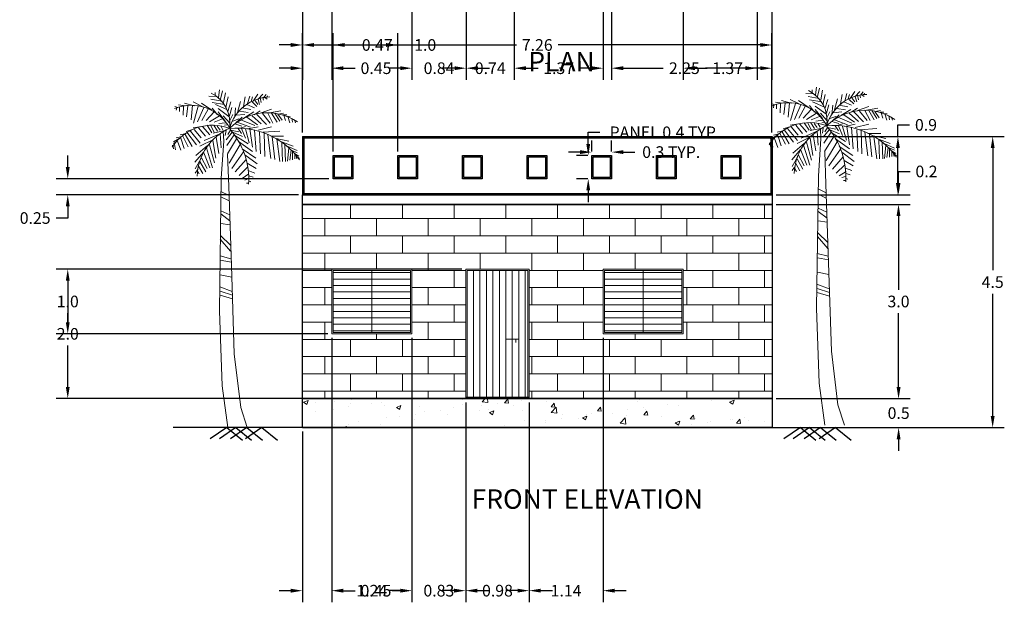
# Model space of a CAD drawing. Units: metres. Extents: x 40.9 to 56.1, y -1.4 to 24.2.
# Tile 1 of 7: x 40.9 to 56.1, y -1.4 to 7.6. Entities that reach past the tile are written whole.
import ezdxf

# ---------------------------------------------------------------- set-up
doc = ezdxf.new("R2010")
doc.units = ezdxf.units.M
doc.header["$MEASUREMENT"] = 0
for name, color, linetype, lineweight in [('A-ANNO-DIMS', 2, 'Continuous', 18), ('A-ANNO-TITL', 7, 'Continuous', 25), ('A-ELEV', 7, 'Continuous', 30), ('A-ELEV-DOOR', 3, 'Continuous', 18), ('A-ELEV-GLAZ', 4, 'Continuous', 18), ('A-ELEV-GRND', 7, 'Continuous', 25), ('A-ELEV-PATT', 252, 'Continuous', 13), ('L-PLNT', 94, 'Continuous', 13)]:
    doc.layers.add(name, color=color, linetype=linetype, lineweight=lineweight)
doc.styles.get("Standard").update_dxf_attribs({"font": 'arial.ttf'})
doc.dimstyles.get("Standard").update_dxf_attribs({"dimtxt": 0.18, "dimasz": 0.18, "dimexe": 0.18, "dimexo": 0.0625, "dimgap": 0.09, "dimtad": 0, "dimtih": 1, "dimtoh": 1, "dimdec": 1, "dimzin": 0, "dimdsep": 46, "dimtxsty": 'Standard', "dimcen": 0.09, "dimadec": 0, "dimazin": 0, "dimtfac": 1, "dimtdec": 1, "dimtofl": 0, "dimtmove": 0, "dimatfit": 3, "dimfxl": 1, "dimtolj": 1, "dimtzin": 0, "dimarcsym": 0})

# ---------------------------------------------------------------- blocks, each defined once
blk = doc.blocks.new('*U47')
for p, q in [((-190.5, 5071.872), (-190.5, 5027.8284)), ((-141.4018, 4996.3578), (-126.6698, 5109.6418)), ((-111.9378, 4971.1864), (-82.4738, 5097.0688)), ((-386.8928, 4857.877), (-524.3576, 4927.1174)), ((-170.8658, 5008.9308), (-288.6964, 5015.23)), ((-87.4014, 4939.7158), (-254.3302, 4971.1864)), ((-48.1076, 4889.3476), (-234.696, 4920.8182)), ((-62.8396, 4920.8182), (-33.401, 5065.5982)), ((-28.4734, 4845.2786), (5.8928, 5002.657)), ((0.9652, 4782.3374), (45.1612, 4927.1174)), ((148.2598, 4769.7644), (192.4558, 4933.4166)), ((236.6518, 4857.877), (261.1882, 5002.657)), ((300.4566, 4901.946), (334.8228, 5015.23)), ((354.4824, 4933.4166), (374.1166, 5002.657)), ((369.2144, 4927.1174), (437.9468, 4857.877)), ((383.9464, 4939.7158), (452.6788, 5046.7006)), ((408.4828, 4952.2888), (452.6788, 4889.3476)), ((457.581, 4971.1864), (531.2156, 5046.7006)), ((457.581, 4964.8872), (482.1174, 4889.3476)), ((491.9472, 4990.0586), (506.6792, 4920.8182)), ((531.2156, 4990.0586), (541.0454, 4952.2888)), ((541.0454, 4990.0586), (580.3138, 5040.4014)), ((560.6796, 4996.3578), (595.0458, 4971.1864)), ((590.1436, 4996.3578), (599.948, 5021.5292)), ((-755.1166, 4845.2786), (-799.3126, 4857.877)), ((-769.8486, 4839.0048), (-779.653, 4801.235)), ((-642.1882, 4870.4754), (-745.2868, 4883.0484)), ((-730.5802, 4845.2786), (-730.5802, 4782.3374)), ((-671.6522, 4864.1762), (-676.5544, 4725.6954)), ((-509.6256, 4870.4754), (-656.9202, 4908.2452)), ((-602.9198, 4870.4754), (-622.554, 4700.524)), ((-534.1874, 4876.7492), (-553.8216, 4656.455)), ((-445.7954, 4864.1762), (-519.4554, 4606.1122)), ((-362.331, 4845.2786), (-460.5274, 4624.9844)), ((-239.5982, 4801.235), (-396.6972, 4908.2452)), ((-298.5262, 4820.1072), (-391.795, 4643.882)), ((-205.232, 4776.0636), (-327.9648, 4643.882)), ((-156.1338, 4731.9946), (-234.696, 4832.7056)), ((-13.7414, 4813.808), (-185.5978, 4889.3476)), ((-146.304, 4826.4064), (15.6972, 4706.8232)), ((-146.304, 4776.0636), (-38.3032, 4637.5828)), ((25.527, 4719.3962), (59.8932, 4845.2786)), ((104.0892, 4700.524), (118.8212, 4839.0048)), ((177.7238, 4788.6366), (310.2864, 4769.7644)), ((217.0176, 4839.0048), (349.5802, 4813.808)), ((241.554, 4681.6518), (393.7508, 4776.0636)), ((285.75, 4889.3476), (403.5806, 4839.0048)), ((398.653, 4731.9946), (491.9472, 4794.9358)), ((491.9472, 4757.166), (663.7782, 4820.1072)), ((629.412, 4763.4652), (801.2684, 4794.9358)), ((-126.6698, 4719.3962), (-278.8666, 4624.9844)), ((-82.4738, 4669.0534), (-205.232, 4618.6852)), ((-67.7672, 4719.3962), (30.4292, 4606.1122)), ((25.527, 4637.5828), (74.6252, 4738.2938)), ((74.6252, 4637.5828), (167.894, 4669.0534)), ((123.7234, 4725.6954), (256.286, 4738.2938)), ((123.7234, 4612.4114), (217.0176, 4694.2248)), ((143.3576, 4618.6852), (344.6526, 4543.171)), ((197.358, 4656.455), (408.4828, 4568.3424)), ((285.75, 4694.2248), (447.7512, 4580.9408)), ((369.2144, 4719.3962), (506.6792, 4593.5138)), ((437.9468, 4738.2938), (585.2414, 4587.2146)), ((526.3134, 4750.8668), (639.2418, 4606.1122)), ((604.8756, 4757.166), (683.4378, 4606.1122)), ((663.7782, 4757.166), (747.2426, 4618.6852)), ((712.8764, 4757.166), (786.5364, 4637.5828)), ((757.0724, 4744.593), (820.9026, 4650.1812)), ((761.9746, 4744.593), (840.5368, 4757.166)), ((825.8048, 4731.9946), (894.5372, 4731.9946)), ((850.3666, 4725.6954), (874.903, 4643.882)), ((904.367, 4713.1224), (943.6354, 4706.8232)), ((909.2692, 4706.8232), (938.7332, 4612.4114)), ((968.1972, 4681.6518), (978.0016, 4618.6852)), ((1012.3678, 4643.882), (1022.1976, 4612.4114)), ((-534.1874, 4511.7004), (-632.3838, 4480.2298)), ((-563.6514, 4486.529), (-416.3314, 4303.9792)), ((-396.6972, 4555.744), (-524.3576, 4536.8718)), ((-509.6256, 4511.7004), (-401.6248, 4385.818)), ((-440.8932, 4536.8718), (-337.7946, 4410.9894)), ((-381.9652, 4555.744), (-273.9644, 4429.8616)), ((-313.2328, 4574.6416), (-239.5982, 4461.3322)), ((-259.2324, 4574.6416), (-205.232, 4467.6314)), ((-43.2054, 4492.8028), (-219.964, 4455.0584)), ((-210.1342, 4574.6416), (-156.1338, 4486.529)), ((-161.036, 4562.0432), (-116.84, 4499.102)), ((-33.401, 4612.4114), (-136.4996, 4599.813)), ((-102.1334, 4555.744), (-72.6694, 4505.4012)), ((-67.7672, 4480.2298), (-60.3504, 4333.0876)), ((-8.8392, 4580.9408), (-48.1076, 4574.6416)), ((-23.5712, 4492.8028), (-38.3032, 4417.2886)), ((40.259, 4499.102), (0.9652, 4436.1608)), ((40.259, 4499.102), (167.894, 4473.9306)), ((104.0892, 4593.5138), (212.09, 4562.0432)), ((158.0896, 4524.2734), (207.1878, 4448.7592)), ((187.5536, 4530.5726), (266.0904, 4555.744)), ((207.1878, 4524.2734), (266.0904, 4379.5188)), ((266.0904, 4517.9996), (325.0184, 4310.2784)), ((300.4566, 4517.9996), (457.581, 4549.4702)), ((334.8228, 4517.9996), (374.1166, 4241.038)), ((403.5806, 4499.102), (428.117, 4178.0968)), ((457.581, 4499.102), (663.7782, 4549.4702)), ((531.2156, 4467.6314), (786.5364, 4486.529)), ((-735.4824, 4373.2196), (-823.849, 4322.8768)), ((-696.1886, 4404.6902), (-779.653, 4385.818)), ((-760.0188, 4335.4498), (-710.9206, 4196.969)), ((-637.286, 4448.7592), (-720.7504, 4429.8616)), ((-710.9206, 4379.5188), (-661.8224, 4222.1658)), ((-681.4566, 4410.9894), (-598.0176, 4247.3372)), ((-647.0904, 4436.1608), (-539.0896, 4253.6364)), ((-617.6518, 4467.6314), (-475.2594, 4278.8078)), ((-215.0364, 4360.6212), (-421.259, 4259.9102)), ((-107.0356, 4448.7592), (-357.4288, 4341.749)), ((-224.8662, 4341.749), (-180.6702, 4077.3858)), ((-175.768, 4392.0918), (-136.4996, 4146.6262)), ((-116.84, 4442.46), (-102.1334, 4234.7388)), ((64.7954, 4467.6314), (-23.5712, 4354.3474)), ((94.2594, 4429.8616), (-13.7414, 4266.2094)), ((133.5278, 4366.9204), (-3.937, 4140.327)), ((74.6252, 4467.6314), (221.9198, 4404.6902)), ((108.9914, 4417.2886), (310.2864, 4291.4062)), ((162.9918, 4329.1506), (374.1166, 4178.0968)), ((482.1174, 4467.6314), (496.8494, 4140.327)), ((550.8752, 4455.0584), (560.6796, 4102.5572)), ((604.8756, 4429.8616), (649.0716, 4071.0866)), ((649.0716, 4410.9894), (845.439, 4410.9894)), ((673.608, 4398.391), (712.8764, 4058.5136)), ((732.5106, 4373.2196), (924.0012, 4335.4498)), ((742.3404, 4366.9204), (786.5364, 4027.043)), ((786.5364, 4335.4498), (987.8314, 4259.9102)), ((-828.7512, 4266.2094), (-843.4832, 4266.2094)), ((-828.7512, 4259.9102), (-823.849, 4215.8666)), ((-789.4828, 4316.5776), (-823.849, 4297.68)), ((-804.2148, 4285.107), (-789.4828, 4203.2682)), ((-362.331, 4171.7976), (-499.8212, 4014.4446)), ((-308.3306, 4266.2094), (-485.0892, 4115.1556)), ((-323.0626, 4234.7388), (-229.7684, 3932.6312)), ((-278.8666, 4278.8078), (-200.3298, 4008.1454)), ((187.5536, 4285.107), (20.6248, 4001.8462)), ((236.6518, 4171.7976), (59.8932, 3920.0328)), ((217.0176, 4215.8666), (423.2148, 4077.3858)), ((816.0004, 4310.2784), (825.8048, 4027.043)), ((865.0732, 4285.107), (874.903, 4027.043)), ((899.4648, 4259.9102), (1051.6616, 4190.6952)), ((924.0012, 4228.4396), (904.367, 4033.3168)), ((958.3674, 4196.969), (938.7332, 4045.9152)), ((963.2696, 4196.969), (1051.6616, 4159.2246)), ((978.0016, 4178.0968), (978.0016, 4052.2144)), ((-406.527, 4064.7874), (-494.8936, 3913.7336)), ((-421.259, 4027.043), (-332.8924, 3869.69)), ((-396.6972, 4083.685), (-313.2328, 3920.0328)), ((-362.331, 4159.2246), (-273.9644, 3932.6312)), ((275.9202, 4058.5136), (113.8936, 3869.69)), ((256.286, 4127.754), (442.849, 3989.2732)), ((1007.4656, 4146.6262), (1076.198, 4108.8564)), ((1012.3678, 4134.0278), (1012.3678, 4064.7874)), ((1036.9296, 4108.8564), (1046.734, 4064.7874)), ((1046.734, 4102.5572), (1086.0278, 4071.0866)), ((-460.5274, 3901.1606), (-494.8936, 3850.7924)), ((-455.6252, 3875.9638), (-431.0888, 3838.2194)), ((-440.8932, 3957.8026), (-377.063, 3844.4932)), ((300.4566, 3938.905), (172.8216, 3813.0226)), ((290.6522, 4001.8462), (428.117, 3920.0328)), ((310.2864, 3888.5622), (408.4828, 3850.7924)), ((320.1162, 3838.2194), (217.0176, 3768.979)), ((310.2864, 3762.6798), (256.286, 3743.7822)), ((315.1886, 3731.2092), (349.5802, 3718.6108)), ((320.1162, 3806.7488), (383.9464, 3787.8512)), ((315.1886, 3699.7386), (280.8224, 3699.7386)), ((-103.6574, 3572.383), (19.1262, 3511.8294)), ((-103.6574, 3493.6938), (19.1262, 3433.1402)), ((-103.6574, 3281.807), (28.5496, 3221.2534)), ((-103.6574, 3233.3692), (33.274, 3130.4484)), ((-103.6574, 3088.0812), (33.274, 3069.9202)), ((-113.1062, 2851.9882), (42.7228, 2670.3782)), ((-108.3818, 2906.4712), (42.7228, 2761.1832)), ((-117.8306, 2597.7342), (47.4472, 2555.3416)), ((-113.1062, 2531.1354), (56.896, 2500.8586)), ((-113.1062, 2313.2034), (61.6204, 2276.8814)), ((-122.555, 2131.5934), (66.3448, 2058.9494)), ((-117.8306, 2064.9946), (71.0438, 2004.4664)), ((-117.8306, 2004.4664), (71.0438, 1949.9834))]:
    blk.add_line(p, q)
for points in [[(-60.0202, 4332.0462), (-98.552, 3772.027), (-126.6952, 1768.7036), (-84.455, 631.6726), (0, 0)], [(-2.9464, 4136.3392), (14.0716, 3645.7128), (56.3118, 2454.529), (98.552, 1118.9716), (197.104, 306.8066), (295.656, 0)]]:
    blk.add_lwpolyline(points)
for centre, radius, start, end in [((-468.0458, 4608.7792), 500.7615, 350.285, 64.11229), ((650.113, 4357.8018), 645.0437, 91.40319, 163.882), ((-552.1452, 4218.7876), 657.8234, 27.67115, 112.5305), ((601.6498, 3945.6614), 817.5767, 56.19272, 134.3213), ((-235.1786, 3853.9928), 721.0064, 68.38311, 147.5322), ((365.6076, 3769.1822), 831.8901, 113.7592, 177.4133), ((148.0312, 3371.0372), 1159.2273, 35.98777, 95.82273), ((-833.12, 3757.2442), 1150.8562, 356.1943, 41.37848)]:
    blk.add_arc(centre, radius, start, end)
blk = doc.blocks.new('*D48')
at = {"layer": 'A-ANNO-DIMS', "color": 0, "lineweight": -2, "transparency": 16777216}
for p, q in [((54.473, 1.933), (54.473, 2.113)), ((52.578, 1.753), (54.653, 1.753)), ((52.578, 1.303), (54.653, 1.303)), ((54.473, 1.123), (54.473, 0.943))]:
    blk.add_line(p, q, dxfattribs=at)
at = {"layer": 'A-ANNO-DIMS', "color": 0, "transparency": 16777216}
for points in [[(54.443, 1.933), (54.503, 1.933), (54.473, 1.753)], [(54.443, 1.123), (54.503, 1.123), (54.473, 1.303)]]:
    blk.add_solid(points, dxfattribs=at)
at = {"layer": 'Defpoints', "color": 0, "transparency": 16777216}
for p in [(52.515, 1.753), (52.515, 1.303), (54.473, 1.303)]:
    blk.add_point(p, dxfattribs=at)
at = {"layer": 'A-ANNO-DIMS', "color": 0, "transparency": 16777216, "insert": (54.473, 1.528), "char_height": 0.18, "attachment_point": 5}
blk.add_mtext('\\A1;0.5', dxfattribs=at)
blk = doc.blocks.new('*D49')
at = {"layer": 'A-ANNO-DIMS', "color": 0, "lineweight": -2, "transparency": 16777216}
for p, q in [((52.578, 4.753), (54.651, 4.753)), ((54.471, 4.573), (54.471, 3.435)), ((54.471, 1.933), (54.471, 3.071)), ((52.578, 1.753), (54.651, 1.753))]:
    blk.add_line(p, q, dxfattribs=at)
at = {"layer": 'A-ANNO-DIMS', "color": 0, "transparency": 16777216}
for points in [[(54.441, 4.573), (54.501, 4.573), (54.471, 4.753)], [(54.441, 1.933), (54.501, 1.933), (54.471, 1.753)]]:
    blk.add_solid(points, dxfattribs=at)
at = {"layer": 'Defpoints', "color": 0, "transparency": 16777216}
for p in [(52.515, 4.753), (54.471, 4.753), (52.515, 1.753)]:
    blk.add_point(p, dxfattribs=at)
at = {"layer": 'A-ANNO-DIMS', "color": 0, "transparency": 16777216, "insert": (54.471, 3.253), "char_height": 0.18, "attachment_point": 5}
blk.add_mtext('\\A1;3.0', dxfattribs=at)
blk = doc.blocks.new('*D50')
at = {"layer": 'A-ANNO-DIMS', "color": 0, "lineweight": -2, "transparency": 16777216}
for p, q in [((54.471, 5.083), (54.471, 5.263)), ((54.471, 5.263), (54.651, 5.263)), ((52.578, 4.903), (54.651, 4.903)), ((52.578, 4.753), (54.651, 4.753)), ((54.471, 4.573), (54.471, 4.393))]:
    blk.add_line(p, q, dxfattribs=at)
at = {"layer": 'A-ANNO-DIMS', "color": 0, "transparency": 16777216}
for points in [[(54.441, 5.083), (54.501, 5.083), (54.471, 4.903)], [(54.441, 4.573), (54.501, 4.573), (54.471, 4.753)]]:
    blk.add_solid(points, dxfattribs=at)
at = {"layer": 'Defpoints', "color": 0, "transparency": 16777216}
for p in [(52.515, 4.903), (54.471, 4.903), (52.515, 4.753)]:
    blk.add_point(p, dxfattribs=at)
at = {"layer": 'A-ANNO-DIMS', "color": 0, "transparency": 16777216, "insert": (54.904, 5.263), "char_height": 0.18, "attachment_point": 5}
blk.add_mtext('\\A1;0.2', dxfattribs=at)
blk = doc.blocks.new('*D51')
at = {"layer": 'A-ANNO-DIMS', "color": 0, "lineweight": -2, "transparency": 16777216}
for p, q in [((54.462, 5.803), (54.462, 5.983)), ((54.462, 5.983), (54.642, 5.983)), ((52.578, 5.803), (54.642, 5.803)), ((54.462, 5.083), (54.462, 5.623)), ((52.578, 4.903), (54.642, 4.903))]:
    blk.add_line(p, q, dxfattribs=at)
at = {"layer": 'A-ANNO-DIMS', "color": 0, "transparency": 16777216}
for points in [[(54.432, 5.623), (54.492, 5.623), (54.462, 5.803)], [(54.432, 5.083), (54.492, 5.083), (54.462, 4.903)]]:
    blk.add_solid(points, dxfattribs=at)
at = {"layer": 'Defpoints', "color": 0, "transparency": 16777216}
for p in [(52.515, 5.803), (54.462, 5.803), (52.515, 4.903)]:
    blk.add_point(p, dxfattribs=at)
at = {"layer": 'A-ANNO-DIMS', "color": 0, "transparency": 16777216, "insert": (54.896, 5.983), "char_height": 0.18, "attachment_point": 5}
blk.add_mtext('\\A1;0.9', dxfattribs=at)
blk = doc.blocks.new('PARAPET-FRAMED-PANEL')
for points in [[(0, 0.358), (0.306, 0.358), (0.306, 0), (0, 0)], [(0.02, 0.338), (0.286, 0.338), (0.286, 0.02), (0.02, 0.02)]]:
    blk.add_lwpolyline(points, close=True)
blk = doc.blocks.new('GRADE-MARK-ELEV')
for p, q in [((0.255, 0.195), (0, 0.02)), ((0.396, 0.195), (0.141, 0.02)), ((0.255, 0.195), (0.496, 0)), ((0.566, 0.195), (0.311, 0.02)), ((0.396, 0.195), (0.637, 0)), ((0.799, 0.195), (0.544, 0.02)), ((0.566, 0.195), (0.807, 0)), ((0.799, 0.195), (1.04, 0))]:
    blk.add_line(p, q)
blk = doc.blocks.new('*D77')
at = {"layer": 'A-ANNO-DIMS', "color": 0, "lineweight": -2, "transparency": 16777216}
for p, q in [((49.674, 5.688), (49.674, 5.868)), ((49.674, 5.868), (49.854, 5.868)), ((49.665, 5.508), (49.494, 5.508)), ((49.665, 5.15), (49.494, 5.15)), ((49.674, 4.97), (49.674, 4.79))]:
    blk.add_line(p, q, dxfattribs=at)
at = {"layer": 'A-ANNO-DIMS', "color": 0, "transparency": 16777216}
for points in [[(49.644, 5.688), (49.704, 5.688), (49.674, 5.508)], [(49.644, 4.97), (49.704, 4.97), (49.674, 5.15)]]:
    blk.add_solid(points, dxfattribs=at)
at = {"layer": 'Defpoints', "color": 0, "transparency": 16777216}
for p in [(49.674, 5.508), (49.728, 5.508), (49.728, 5.15)]:
    blk.add_point(p, dxfattribs=at)
at = {"layer": 'A-ANNO-DIMS', "color": 0, "transparency": 16777216, "insert": (50.86, 5.868), "char_height": 0.18, "attachment_point": 5}
blk.add_mtext('\\A1;PANEL 0.4 TYP.', dxfattribs=at)
blk = doc.blocks.new('*D78')
at = {"layer": 'A-ANNO-DIMS', "color": 0, "lineweight": -2, "transparency": 16777216}
for p, q in [((49.728, 5.57), (49.728, 5.742)), ((50.034, 5.57), (50.034, 5.742)), ((49.548, 5.562), (49.368, 5.562)), ((50.214, 5.562), (50.394, 5.562))]:
    blk.add_line(p, q, dxfattribs=at)
at = {"layer": 'A-ANNO-DIMS', "color": 0, "transparency": 16777216}
for points in [[(49.548, 5.592), (49.548, 5.532), (49.728, 5.562)], [(50.214, 5.592), (50.214, 5.532), (50.034, 5.562)]]:
    blk.add_solid(points, dxfattribs=at)
at = {"layer": 'Defpoints', "color": 0, "transparency": 16777216}
for p in [(49.728, 5.508), (50.034, 5.562), (50.034, 5.508)]:
    blk.add_point(p, dxfattribs=at)
at = {"layer": 'A-ANNO-DIMS', "color": 0, "transparency": 16777216, "insert": (50.957, 5.562), "char_height": 0.18, "attachment_point": 5}
blk.add_mtext('\\A1;0.3 TYP.', dxfattribs=at)
blk = doc.blocks.new('*D117')
at = {"layer": 'A-ANNO-DIMS', "color": 0, "lineweight": -2, "transparency": 16777216}
for p, q in [((45.255, 5.866), (45.255, 7.398)), ((52.515, 5.866), (52.515, 7.398)), ((45.435, 7.218), (48.562, 7.218)), ((52.335, 7.218), (49.208, 7.218))]:
    blk.add_line(p, q, dxfattribs=at)
at = {"layer": 'A-ANNO-DIMS', "color": 0, "transparency": 16777216}
for points in [[(45.435, 7.248), (45.435, 7.188), (45.255, 7.218)], [(52.335, 7.248), (52.335, 7.188), (52.515, 7.218)]]:
    blk.add_solid(points, dxfattribs=at)
at = {"layer": 'Defpoints', "color": 0, "transparency": 16777216}
for p in [(52.515, 7.218), (45.255, 5.803), (52.515, 5.803)]:
    blk.add_point(p, dxfattribs=at)
at = {"layer": 'A-ANNO-DIMS', "color": 0, "transparency": 16777216, "insert": (48.885, 7.218), "char_height": 0.18, "attachment_point": 5}
blk.add_mtext('\\A1;7.26', dxfattribs=at)
blk = doc.blocks.new('*D118')
at = {"layer": 'A-ANNO-DIMS', "color": 0, "lineweight": -2, "transparency": 16777216}
for p, q in [((52.578, 5.803), (56.107, 5.803)), ((55.927, 5.623), (55.927, 3.735)), ((55.927, 1.483), (55.927, 3.371)), ((52.578, 1.303), (56.107, 1.303))]:
    blk.add_line(p, q, dxfattribs=at)
at = {"layer": 'A-ANNO-DIMS', "color": 0, "transparency": 16777216}
for points in [[(55.897, 5.623), (55.957, 5.623), (55.927, 5.803)], [(55.897, 1.483), (55.957, 1.483), (55.927, 1.303)]]:
    blk.add_solid(points, dxfattribs=at)
at = {"layer": 'Defpoints', "color": 0, "transparency": 16777216}
for p in [(52.515, 5.803), (55.927, 5.803), (52.515, 1.303)]:
    blk.add_point(p, dxfattribs=at)
at = {"layer": 'A-ANNO-DIMS', "color": 0, "transparency": 16777216, "insert": (55.927, 3.553), "char_height": 0.18, "attachment_point": 5}
blk.add_mtext('\\A1;4.5', dxfattribs=at)
blk = doc.blocks.new('*D119')
at = {"layer": 'A-ANNO-DIMS', "color": 0, "lineweight": -2, "transparency": 16777216}
for p, q in [((45.708, 2.691), (45.708, -1.397)), ((45.255, 1.241), (45.255, -1.397)), ((45.075, -1.217), (44.895, -1.217)), ((45.888, -1.217), (46.068, -1.217))]:
    blk.add_line(p, q, dxfattribs=at)
at = {"layer": 'A-ANNO-DIMS', "color": 0, "transparency": 16777216}
for points in [[(45.075, -1.187), (45.075, -1.247), (45.255, -1.217)], [(45.888, -1.187), (45.888, -1.247), (45.708, -1.217)]]:
    blk.add_solid(points, dxfattribs=at)
at = {"layer": 'Defpoints', "color": 0, "transparency": 16777216}
for p in [(45.708, 2.753), (45.255, 1.303), (45.708, -1.217)]:
    blk.add_point(p, dxfattribs=at)
at = {"layer": 'A-ANNO-DIMS', "color": 0, "transparency": 16777216, "insert": (46.392, -1.217), "char_height": 0.18, "attachment_point": 5}
blk.add_mtext('\\A1;0.45', dxfattribs=at)
blk = doc.blocks.new('*D120')
at = {"layer": 'A-ANNO-DIMS', "color": 0, "lineweight": -2, "transparency": 16777216}
for p, q in [((45.708, 2.691), (45.708, -1.397)), ((46.948, 2.691), (46.948, -1.397)), ((45.888, -1.217), (46.013, -1.217)), ((46.768, -1.217), (46.642, -1.217))]:
    blk.add_line(p, q, dxfattribs=at)
at = {"layer": 'A-ANNO-DIMS', "color": 0, "transparency": 16777216}
for points in [[(45.888, -1.187), (45.888, -1.247), (45.708, -1.217)], [(46.768, -1.187), (46.768, -1.247), (46.948, -1.217)]]:
    blk.add_solid(points, dxfattribs=at)
at = {"layer": 'Defpoints', "color": 0, "transparency": 16777216}
for p in [(45.708, 2.753), (46.948, 2.753), (46.948, -1.217)]:
    blk.add_point(p, dxfattribs=at)
at = {"layer": 'A-ANNO-DIMS', "color": 0, "transparency": 16777216, "insert": (46.328, -1.217), "char_height": 0.18, "attachment_point": 5}
blk.add_mtext('\\A1;1.24', dxfattribs=at)
blk = doc.blocks.new('*D121')
at = {"layer": 'A-ANNO-DIMS', "color": 0, "lineweight": -2, "transparency": 16777216}
for p, q in [((46.947505, 2.690529), (46.947505, -1.396719)), ((47.780203, 1.690529), (47.780203, -1.396719)), ((46.767505, -1.216719), (46.587505, -1.216719)), ((47.960203, -1.216719), (48.140203, -1.216719))]:
    blk.add_line(p, q, dxfattribs=at)
at = {"layer": 'A-ANNO-DIMS', "color": 0, "transparency": 16777216}
for points in [[(46.767505, -1.186719), (46.767505, -1.246719), (46.947505, -1.216719)], [(47.960203, -1.186719), (47.960203, -1.246719), (47.780203, -1.216719)]]:
    blk.add_solid(points, dxfattribs=at)
at = {"layer": 'Defpoints', "color": 0, "transparency": 16777216}
for p in [(46.947505, 2.753029), (47.780203, 1.753029), (47.780203, -1.216719)]:
    blk.add_point(p, dxfattribs=at)
at = {"layer": 'A-ANNO-DIMS', "color": 0, "transparency": 16777216, "insert": (47.363854, -1.216719), "char_height": 0.18, "attachment_point": 5}
blk.add_mtext('\\A1;0.83', dxfattribs=at)
blk = doc.blocks.new('*D122')
at = {"layer": 'A-ANNO-DIMS', "color": 0, "lineweight": -2, "transparency": 16777216}
for p, q in [((47.780203, 1.690529), (47.780203, -1.396719)), ((48.760203, 1.690529), (48.760203, -1.396719)), ((47.600203, -1.216719), (47.420203, -1.216719)), ((48.940203, -1.216719), (49.120203, -1.216719))]:
    blk.add_line(p, q, dxfattribs=at)
at = {"layer": 'A-ANNO-DIMS', "color": 0, "transparency": 16777216}
for points in [[(47.600203, -1.186719), (47.600203, -1.246719), (47.780203, -1.216719)], [(48.940203, -1.186719), (48.940203, -1.246719), (48.760203, -1.216719)]]:
    blk.add_solid(points, dxfattribs=at)
at = {"layer": 'Defpoints', "color": 0, "transparency": 16777216}
for p in [(47.780203, 1.753029), (48.760203, 1.753029), (48.760203, -1.216719)]:
    blk.add_point(p, dxfattribs=at)
at = {"layer": 'A-ANNO-DIMS', "color": 0, "transparency": 16777216, "insert": (48.270203, -1.216719), "char_height": 0.18, "attachment_point": 5}
blk.add_mtext('\\A1;0.98', dxfattribs=at)
blk = doc.blocks.new('*D123')
at = {"layer": 'A-ANNO-DIMS', "color": 0, "lineweight": -2, "transparency": 16777216}
for p, q in [((49.902703, 2.690529), (49.902703, -1.396719)), ((48.760203, 1.690529), (48.760203, -1.396719)), ((48.580203, -1.216719), (48.400203, -1.216719)), ((50.082703, -1.216719), (50.262703, -1.216719))]:
    blk.add_line(p, q, dxfattribs=at)
at = {"layer": 'A-ANNO-DIMS', "color": 0, "transparency": 16777216}
for points in [[(48.580203, -1.186719), (48.580203, -1.246719), (48.760203, -1.216719)], [(50.082703, -1.186719), (50.082703, -1.246719), (49.902703, -1.216719)]]:
    blk.add_solid(points, dxfattribs=at)
at = {"layer": 'Defpoints', "color": 0, "transparency": 16777216}
for p in [(49.902703, 2.753029), (48.760203, 1.753029), (49.902703, -1.216719)]:
    blk.add_point(p, dxfattribs=at)
at = {"layer": 'A-ANNO-DIMS', "color": 0, "transparency": 16777216, "insert": (49.331453, -1.216719), "char_height": 0.18, "attachment_point": 5}
blk.add_mtext('\\A1;1.14', dxfattribs=at)
blk = doc.blocks.new('*D124')
at = {"layer": 'A-ANNO-DIMS', "color": 0, "lineweight": -2, "transparency": 16777216}
for p, q in [((45.645, 3.753), (41.446, 3.753)), ((41.626, 3.573), (41.626, 3.435)), ((41.626, 2.933), (41.626, 3.071)), ((45.645, 2.753), (41.446, 2.753))]:
    blk.add_line(p, q, dxfattribs=at)
at = {"layer": 'A-ANNO-DIMS', "color": 0, "transparency": 16777216}
for points in [[(41.596, 3.573), (41.656, 3.573), (41.626, 3.753)], [(41.596, 2.933), (41.656, 2.933), (41.626, 2.753)]]:
    blk.add_solid(points, dxfattribs=at)
at = {"layer": 'Defpoints', "color": 0, "transparency": 16777216}
for p in [(41.626, 3.753), (45.708, 3.753), (45.708, 2.753)]:
    blk.add_point(p, dxfattribs=at)
at = {"layer": 'A-ANNO-DIMS', "color": 0, "transparency": 16777216, "insert": (41.626, 3.253), "char_height": 0.18, "attachment_point": 5}
blk.add_mtext('\\A1;1.0', dxfattribs=at)
blk = doc.blocks.new('*D125')
at = {"layer": 'A-ANNO-DIMS', "color": 0, "lineweight": -2, "transparency": 16777216}
for p, q in [((47.718, 3.753), (41.446, 3.753)), ((41.626, 3.573), (41.626, 2.935)), ((41.626, 1.933), (41.626, 2.571)), ((47.718, 1.753), (41.446, 1.753))]:
    blk.add_line(p, q, dxfattribs=at)
at = {"layer": 'A-ANNO-DIMS', "color": 0, "transparency": 16777216}
for points in [[(41.596, 3.573), (41.656, 3.573), (41.626, 3.753)], [(41.596, 1.933), (41.656, 1.933), (41.626, 1.753)]]:
    blk.add_solid(points, dxfattribs=at)
at = {"layer": 'Defpoints', "color": 0, "transparency": 16777216}
for p in [(41.626, 3.753), (47.78, 3.753), (47.78, 1.753)]:
    blk.add_point(p, dxfattribs=at)
at = {"layer": 'A-ANNO-DIMS', "color": 0, "transparency": 16777216, "insert": (41.626, 2.753), "char_height": 0.18, "attachment_point": 5}
blk.add_mtext('\\A1;2.0', dxfattribs=at)
blk = doc.blocks.new('*D126')
at = {"layer": 'A-ANNO-DIMS', "color": 0, "lineweight": -2, "transparency": 16777216}
for p, q in [((45.255, 5.866), (45.255, 7.398)), ((45.728, 5.57), (45.728, 7.398)), ((45.075, 7.218), (44.895, 7.218)), ((45.908, 7.218), (46.088, 7.218))]:
    blk.add_line(p, q, dxfattribs=at)
at = {"layer": 'A-ANNO-DIMS', "color": 0, "transparency": 16777216}
for points in [[(45.075, 7.248), (45.075, 7.188), (45.255, 7.218)], [(45.908, 7.248), (45.908, 7.188), (45.728, 7.218)]]:
    blk.add_solid(points, dxfattribs=at)
at = {"layer": 'Defpoints', "color": 0, "transparency": 16777216}
for p in [(45.728, 7.218), (45.255, 5.803), (45.728, 5.508)]:
    blk.add_point(p, dxfattribs=at)
at = {"layer": 'A-ANNO-DIMS', "color": 0, "transparency": 16777216, "insert": (46.412, 7.218), "char_height": 0.18, "attachment_point": 5}
blk.add_mtext('\\A1;0.47', dxfattribs=at)
blk = doc.blocks.new('*D127')
at = {"layer": 'A-ANNO-DIMS', "color": 0, "lineweight": -2, "transparency": 16777216}
for p, q in [((45.728, 5.57), (45.728, 7.398)), ((46.728, 5.57), (46.728, 7.398)), ((45.908, 7.218), (46.548, 7.218)), ((46.728, 7.218), (46.908, 7.218))]:
    blk.add_line(p, q, dxfattribs=at)
at = {"layer": 'A-ANNO-DIMS', "color": 0, "transparency": 16777216}
for points in [[(45.908, 7.248), (45.908, 7.188), (45.728, 7.218)], [(46.548, 7.248), (46.548, 7.188), (46.728, 7.218)]]:
    blk.add_solid(points, dxfattribs=at)
at = {"layer": 'Defpoints', "color": 0, "transparency": 16777216}
for p in [(46.728, 7.218), (45.728, 5.508), (46.728, 5.508)]:
    blk.add_point(p, dxfattribs=at)
at = {"layer": 'A-ANNO-DIMS', "color": 0, "transparency": 16777216, "insert": (47.153, 7.218), "char_height": 0.18, "attachment_point": 5}
blk.add_mtext('\\A1;1.0', dxfattribs=at)
blk = doc.blocks.new('*D128')
at = {"layer": 'A-ANNO-DIMS', "color": 0, "lineweight": -2, "transparency": 16777216}
for p, q in [((41.626, 5.33), (41.626, 5.51)), ((45.665, 5.15), (41.446, 5.15)), ((45.193, 4.903), (41.446, 4.903)), ((41.626, 4.723), (41.626, 4.543)), ((41.626, 4.543), (41.446, 4.543))]:
    blk.add_line(p, q, dxfattribs=at)
at = {"layer": 'A-ANNO-DIMS', "color": 0, "transparency": 16777216}
for points in [[(41.596, 5.33), (41.656, 5.33), (41.626, 5.15)], [(41.596, 4.723), (41.656, 4.723), (41.626, 4.903)]]:
    blk.add_solid(points, dxfattribs=at)
at = {"layer": 'Defpoints', "color": 0, "transparency": 16777216}
for p in [(45.728, 5.15), (41.626, 4.903), (45.255, 4.903)]:
    blk.add_point(p, dxfattribs=at)
at = {"layer": 'A-ANNO-DIMS', "color": 0, "transparency": 16777216, "insert": (41.122, 4.543), "char_height": 0.18, "attachment_point": 5}
blk.add_mtext('\\A1;0.25', dxfattribs=at)
blk = doc.blocks.new('*D129')
at = {"layer": 'A-ANNO-DIMS', "color": 0, "lineweight": -2, "transparency": 16777216}
for p, q in [((51.143, 8.615), (51.143, 6.679)), ((52.515, 8.615), (52.515, 6.679)), ((51.323, 6.859), (51.514, 6.859)), ((52.335, 6.859), (52.144, 6.859))]:
    blk.add_line(p, q, dxfattribs=at)
at = {"layer": 'A-ANNO-DIMS', "color": 0, "transparency": 16777216}
for points in [[(51.323, 6.889), (51.323, 6.829), (51.143, 6.859)], [(52.335, 6.889), (52.335, 6.829), (52.515, 6.859)]]:
    blk.add_solid(points, dxfattribs=at)
at = {"layer": 'Defpoints', "color": 0, "transparency": 16777216}
for p in [(51.143, 8.677), (52.515, 8.677), (52.515, 6.859)]:
    blk.add_point(p, dxfattribs=at)
at = {"layer": 'A-ANNO-DIMS', "color": 0, "transparency": 16777216, "insert": (51.829, 6.859), "char_height": 0.18, "attachment_point": 5}
blk.add_mtext('\\A1;1.37', dxfattribs=at)
blk = doc.blocks.new('*D134')
at = {"layer": 'A-ANNO-DIMS', "color": 0, "lineweight": -2, "transparency": 16777216}
for p, q in [((50.034, 13.095), (50.034, 6.679)), ((52.285, 13.095), (52.285, 6.679)), ((50.214, 6.859), (50.834, 6.859)), ((52.105, 6.859), (51.486, 6.859))]:
    blk.add_line(p, q, dxfattribs=at)
at = {"layer": 'A-ANNO-DIMS', "color": 0, "transparency": 16777216}
for points in [[(50.214, 6.889), (50.214, 6.829), (50.034, 6.859)], [(52.105, 6.889), (52.105, 6.829), (52.285, 6.859)]]:
    blk.add_solid(points, dxfattribs=at)
at = {"layer": 'Defpoints', "color": 0, "transparency": 16777216}
for p in [(50.034, 13.157), (52.285, 13.157), (52.285, 6.859)]:
    blk.add_point(p, dxfattribs=at)
at = {"layer": 'A-ANNO-DIMS', "color": 0, "transparency": 16777216, "insert": (51.16, 6.859), "char_height": 0.18, "attachment_point": 5}
blk.add_mtext('\\A1;2.25', dxfattribs=at)
blk = doc.blocks.new('*D148')
at = {"layer": 'A-ANNO-DIMS', "color": 0, "lineweight": -2, "transparency": 16777216}
for p, q in [((48.53, 8.615), (48.53, 6.679)), ((49.903, 8.615), (49.903, 6.679)), ((48.71, 6.859), (48.901, 6.859)), ((49.723, 6.859), (49.532, 6.859))]:
    blk.add_line(p, q, dxfattribs=at)
at = {"layer": 'A-ANNO-DIMS', "color": 0, "transparency": 16777216}
for points in [[(48.71, 6.889), (48.71, 6.829), (48.53, 6.859)], [(49.723, 6.889), (49.723, 6.829), (49.903, 6.859)]]:
    blk.add_solid(points, dxfattribs=at)
at = {"layer": 'Defpoints', "color": 0, "transparency": 16777216}
for p in [(48.53, 8.677), (49.903, 8.677), (49.903, 6.859)]:
    blk.add_point(p, dxfattribs=at)
at = {"layer": 'A-ANNO-DIMS', "color": 0, "transparency": 16777216, "insert": (49.216, 6.859), "char_height": 0.18, "attachment_point": 5}
blk.add_mtext('\\A1;1.37', dxfattribs=at)
blk = doc.blocks.new('*D149')
at = {"layer": 'A-ANNO-DIMS', "color": 0, "lineweight": -2, "transparency": 16777216}
for p, q in [((45.255, 12.865), (45.255, 6.679)), ((45.708, 12.865), (45.708, 6.679)), ((45.075, 6.859), (44.895, 6.859)), ((45.888, 6.859), (46.068, 6.859))]:
    blk.add_line(p, q, dxfattribs=at)
at = {"layer": 'A-ANNO-DIMS', "color": 0, "transparency": 16777216}
for points in [[(45.075, 6.889), (45.075, 6.829), (45.255, 6.859)], [(45.888, 6.889), (45.888, 6.829), (45.708, 6.859)]]:
    blk.add_solid(points, dxfattribs=at)
at = {"layer": 'Defpoints', "color": 0, "transparency": 16777216}
for p in [(45.255, 12.927), (45.708, 12.927), (45.708, 6.859)]:
    blk.add_point(p, dxfattribs=at)
at = {"layer": 'A-ANNO-DIMS', "color": 0, "transparency": 16777216, "insert": (46.392, 6.859), "char_height": 0.18, "attachment_point": 5}
blk.add_mtext('\\A1;0.45', dxfattribs=at)
blk = doc.blocks.new('*D155')
at = {"layer": 'A-ANNO-DIMS', "color": 0, "lineweight": -2, "transparency": 16777216}
for p, q in [((46.947505, 12.864753), (46.947505, 6.679084)), ((47.786899, 12.864753), (47.786899, 6.679084)), ((46.767505, 6.859084), (46.587505, 6.859084)), ((47.966899, 6.859084), (48.146899, 6.859084))]:
    blk.add_line(p, q, dxfattribs=at)
at = {"layer": 'A-ANNO-DIMS', "color": 0, "transparency": 16777216}
for points in [[(46.767505, 6.889084), (46.767505, 6.829084), (46.947505, 6.859084)], [(47.966899, 6.889084), (47.966899, 6.829084), (47.786899, 6.859084)]]:
    blk.add_solid(points, dxfattribs=at)
at = {"layer": 'Defpoints', "color": 0, "transparency": 16777216}
for p in [(46.947505, 12.927253), (47.786899, 12.927253), (47.786899, 6.859084)]:
    blk.add_point(p, dxfattribs=at)
at = {"layer": 'A-ANNO-DIMS', "color": 0, "transparency": 16777216, "insert": (47.367202, 6.859084), "char_height": 0.18, "attachment_point": 5}
blk.add_mtext('\\A1;0.84', dxfattribs=at)
blk = doc.blocks.new('*D156')
at = {"layer": 'A-ANNO-DIMS', "color": 0, "lineweight": -2, "transparency": 16777216}
for p, q in [((47.786899, 12.864753), (47.786899, 6.679084)), ((48.530203, 12.864753), (48.530203, 6.679084)), ((47.606899, 6.859084), (47.426899, 6.859084)), ((48.710203, 6.859084), (48.890203, 6.859084))]:
    blk.add_line(p, q, dxfattribs=at)
at = {"layer": 'A-ANNO-DIMS', "color": 0, "transparency": 16777216}
for points in [[(47.606899, 6.889084), (47.606899, 6.829084), (47.786899, 6.859084)], [(48.710203, 6.889084), (48.710203, 6.829084), (48.530203, 6.859084)]]:
    blk.add_solid(points, dxfattribs=at)
at = {"layer": 'Defpoints', "color": 0, "transparency": 16777216}
for p in [(47.786899, 12.927253), (48.530203, 12.927253), (48.530203, 6.859084)]:
    blk.add_point(p, dxfattribs=at)
at = {"layer": 'A-ANNO-DIMS', "color": 0, "transparency": 16777216, "insert": (48.158551, 6.859084), "char_height": 0.18, "attachment_point": 5}
blk.add_mtext('\\A1;0.74', dxfattribs=at)

msp = doc.modelspace()

# ---------------------------------------------------------------- hatches: boundary and pattern name
at = {"layer": 'A-ELEV-PATT'}
h = msp.add_hatch(dxfattribs=at)
h.set_pattern_fill('AR-BRSTD', color=256, scale=0.1)
h.paths.add_polyline_path([(52.5152, 4.753), (45.2552, 4.753), (45.2552, 1.753), (47.7802, 1.753), (47.7802, 3.753), (48.7602, 3.753), (48.7602, 1.753), (52.5152, 1.753)])
h.paths.add_polyline_path([(46.9475, 3.753), (46.9475, 2.753), (45.7075, 2.753), (45.7075, 3.753)], flags=16)
h.paths.add_polyline_path([(49.9027, 3.753), (51.1427, 3.753), (51.1427, 2.753), (49.9027, 2.753)], flags=16)
h = msp.add_hatch(dxfattribs=at)
h.set_pattern_fill('_USER', color=256, scale=0.1, pattern_type=0)
h.set_pattern_definition([(0, (0, 0), (0, 0.1), [])])
h.paths.add_polyline_path([(46.9275, 3.733), (45.7275, 3.733), (45.7275, 2.773), (46.9275, 2.773)])
h.paths.add_polyline_path([(51.1227, 3.733), (49.9227, 3.733), (49.9227, 2.773), (51.1227, 2.773)])
h = msp.add_hatch(dxfattribs=at)
h.set_pattern_fill('_USER', color=256, scale=0.1, angle=90, pattern_type=0)
h.set_pattern_definition([(90, (0, 0), (-0.1, 0), [])])
h.paths.add_polyline_path([(48.7402, 3.733), (47.8002, 3.733), (47.8002, 1.773), (48.7402, 1.773)])
h = msp.add_hatch(dxfattribs=at)
h.set_pattern_fill('AR-CONC', color=256, scale=0.1)
h.set_pattern_definition([(50, (0, 0), (0.71726, -0.062752), [0.075, -0.825]), (355, (0, 0), (-0.138751, 0.752192), [0.06, -0.66]), (100.4514, (0.0598, -0.0052), (0.578509, 0.68944), [0.06374, -0.701142]), (46.1842, (0, 0.2), (1.067241, -0.16552), [0.1125, -1.2375]), (96.6356, (0.0889, 0.1862), (0.934662, 0.974119), [0.09561, -1.051714]), (351.1842, (0, 0.2), (0.934662, 0.974119), [0.09, -0.99]), (21, (0.1, 0.15), (0.596907, -0.402619), [0.075, -0.825]), (326, (0.1, 0.15), (0.243315, 0.72515), [0.06, -0.66]), (71.4514, (0.14974, 0.11645), (0.840222, 0.322531), [0.06374, -0.701142]), (37.5, (0, 0), (0.0121599, 0.3328939), [0, -0.652, 0, -0.67, 0, -0.6625]), (7.5, (0, 0), (0.2630695, 0.3944117), [0, -0.382, 0, -0.637, 0, -0.2525]), (327.5, (-0.223, 0), (0.5338224, -0.0225549), [0, -0.25, 0, -0.78, 0, -1.035]), (317.5, (-0.323, 0), (0.583186, 0.100105), [0, -0.325, 0, -0.518, 0, -0.735])])
h.paths.add_polyline_path([(52.5152, 1.753), (45.2552, 1.753), (45.2552, 1.303), (52.5152, 1.303)])

# ---------------------------------------------------------------- linework, layer by layer
at = {"layer": 'A-ELEV'}
for p, q in [((45.2552, 5.803), (52.5152, 5.803)), ((45.2552, 5.803), (45.2552, 4.903)), ((45.2752, 5.803), (45.2752, 4.903)), ((52.4952, 5.803), (52.4952, 4.903)), ((52.5152, 5.803), (52.5152, 4.903)), ((45.2552, 5.783), (52.5152, 5.783)), ((45.2552, 4.923), (52.5152, 4.923)), ((45.2552, 4.903), (52.5152, 4.903)), ((45.2552, 4.903), (52.5152, 4.903)), ((45.2552, 4.753), (52.5152, 4.753)), ((45.2552, 1.753), (52.5152, 1.753)), ((45.2552, 1.303), (52.5152, 1.303))]:
    msp.add_line(p, q, dxfattribs=at)
for points in [[(45.2552, 4.903), (52.5152, 4.903), (52.5152, 4.753), (45.2552, 4.753)], [(45.2552, 4.753), (52.5152, 4.753), (52.5152, 1.753), (45.2552, 1.753)], [(45.2552, 1.753), (52.5152, 1.753), (52.5152, 1.303), (45.2552, 1.303)]]:
    msp.add_lwpolyline(points, close=True, dxfattribs=at)
at = {"layer": 'A-ELEV-DOOR'}
for p, q in [((48.3959, 2.6721), (48.598, 2.6721)), ((48.5521, 2.6721), (48.5521, 2.6207)), ((47.7802, 1.773), (48.7602, 1.773)), ((47.7802, 1.753), (48.7602, 1.753))]:
    msp.add_line(p, q, dxfattribs=at)
for points in [[(47.7802, 3.753), (48.7602, 3.753), (48.7602, 1.753), (47.7802, 1.753)], [(47.8002, 3.733), (48.7402, 3.733), (48.7402, 1.773), (47.8002, 1.773)]]:
    msp.add_lwpolyline(points, close=True, dxfattribs=at)
at = {"layer": 'A-ELEV-GLAZ'}
for p, q in [((46.3275, 3.733), (46.3275, 2.773)), ((50.5227, 3.733), (50.5227, 2.773))]:
    msp.add_line(p, q, dxfattribs=at)
for points in [[(45.7075, 3.753), (46.9475, 3.753), (46.9475, 2.753), (45.7075, 2.753)], [(45.7275, 3.733), (46.9275, 3.733), (46.9275, 2.773), (45.7275, 2.773)], [(49.9027, 3.753), (51.1427, 3.753), (51.1427, 2.753), (49.9027, 2.753)], [(49.9227, 3.733), (51.1227, 3.733), (51.1227, 2.773), (49.9227, 2.773)]]:
    msp.add_lwpolyline(points, close=True, dxfattribs=at)
at = {"layer": 'A-ELEV-GRND'}
for p, q in [((45.2552, 1.303), (43.2552, 1.303)), ((52.5152, 1.303), (54.5152, 1.303))]:
    msp.add_line(p, q, dxfattribs=at)

# ---------------------------------------------------------------- block references
at = {"layer": 'A-ELEV'}
for p in [(45.728, 5.15), (46.728, 5.15), (46.728, 5.15), (47.728, 5.15), (48.728, 5.15), (49.728, 5.15), (50.728, 5.15), (51.728, 5.15)]:
    msp.add_blockref('PARAPET-FRAMED-PANEL', p, dxfattribs=at)
at = {"layer": 'A-ELEV-GRND'}
for p in [(43.8301, 1.108), (52.699, 1.108)]:
    msp.add_blockref('GRADE-MARK-ELEV', p, dxfattribs=at)
at = {"layer": 'L-PLNT', "xscale": 0.0010218072108737, "yscale": 0.0010218072108737, "zscale": 0.0010218072108737}
for p in [(53.3324, 1.3427), (44.1006, 1.303)]:
    msp.add_blockref('*U47', p, dxfattribs=at)

# ---------------------------------------------------------------- texts
at = {"layer": 'A-ANNO-TITL'}
for s, p in [('PLAN', (48.747, 6.8113)), ('FRONT ELEVATION', (47.8709, 0.049))]:
    msp.add_text(s, height=0.3, dxfattribs=at).set_placement(p)

# ---------------------------------------------------------------- dimensions: what is measured, and where the dimension line sits
at = {"layer": 'A-ANNO-DIMS'}
for base, p1, p2, override, picture, middle in [((52.2852, 6.8591), (50.034, 13.1573), (52.2852, 13.1573), {"dimdec": 2, "dimlfac": 1, "dimrnd": 0, "dimzin": 0, "dimdsep": 46, "dimlunit": 2}, '*D134', (51.1596, 6.8591)), ((45.7075, 6.8591), (45.2552, 12.9273), (45.7075, 12.9273), {"dimdec": 2, "dimlfac": 1, "dimrnd": 0, "dimzin": 0, "dimdsep": 46, "dimlunit": 2}, '*D149', (46.392, 6.8591)), ((47.7869, 6.8591), (46.9475, 12.9273), (47.7869, 12.9273), {"dimdec": 2, "dimlfac": 1, "dimrnd": 0, "dimzin": 0, "dimdsep": 46, "dimlunit": 2}, '*D155', (47.3672, 6.8591)), ((48.5302, 6.8591), (47.7869, 12.9273), (48.5302, 12.9273), {"dimdec": 2, "dimlfac": 1, "dimrnd": 0, "dimzin": 0, "dimdsep": 46, "dimlunit": 2}, '*D156', (48.1586, 6.8591)), ((49.9027, 6.8591), (48.5302, 8.6773), (49.9027, 8.6773), {"dimdec": 2, "dimlfac": 1, "dimrnd": 0, "dimzin": 0, "dimdsep": 46, "dimlunit": 2}, '*D148', (49.2165, 6.8591)), ((52.5152, 6.8591), (51.1427, 8.6773), (52.5152, 8.6773), {"dimdec": 2, "dimlfac": 1, "dimrnd": 0, "dimzin": 0, "dimdsep": 46, "dimlunit": 2}, '*D129', (51.829, 6.8591)), ((45.7279, 7.2178), (45.2552, 5.803), (45.7279, 5.5079), {"dimdec": 2, "dimlfac": 1, "dimrnd": 0, "dimzin": 0, "dimdsep": 46, "dimlunit": 2}, '*D126', (46.4117, 7.2178)), ((52.5152, 7.2178), (45.2552, 5.803), (52.5152, 5.803), {"dimdec": 2, "dimlfac": 1, "dimrnd": 0, "dimzin": 0, "dimdsep": 46, "dimlunit": 2}, '*D117', (48.8852, 7.2178)), ((46.7279, 7.2178), (45.7279, 5.5079), (46.7279, 5.5079), {"dimdec": 1, "dimlfac": 1, "dimrnd": 0, "dimzin": 0, "dimdsep": 46, "dimlunit": 2}, '*D127', (47.153, 7.2178)), ((45.7075, -1.2167), (45.2552, 1.303), (45.7075, 2.753), {"dimdec": 2, "dimlfac": 1, "dimrnd": 0, "dimzin": 0, "dimdsep": 46, "dimlunit": 2}, '*D119', (46.392, -1.2167)), ((46.9475, -1.2167), (45.7075, 2.753), (46.9475, 2.753), {"dimdec": 2, "dimlfac": 1, "dimrnd": 0, "dimzin": 0, "dimdsep": 46, "dimlunit": 2}, '*D120', (46.3275, -1.2167)), ((47.7802, -1.2167), (46.9475, 2.753), (47.7802, 1.753), {"dimdec": 2, "dimlfac": 1, "dimrnd": 0, "dimzin": 0, "dimdsep": 46, "dimlunit": 2}, '*D121', (47.3639, -1.2167)), ((49.9027, -1.2167), (48.7602, 1.753), (49.9027, 2.753), {"dimdec": 2, "dimlfac": 1, "dimrnd": 0, "dimzin": 0, "dimdsep": 46, "dimlunit": 2}, '*D123', (49.3315, -1.2167)), ((48.7602, -1.2167), (47.7802, 1.753), (48.7602, 1.753), {"dimdec": 2, "dimlfac": 1, "dimrnd": 0, "dimzin": 0, "dimdsep": 46, "dimlunit": 2}, '*D122', (48.2702, -1.2167))]:
    dim = msp.add_linear_dim(base=base, p1=p1, p2=p2, dimstyle='Standard', override=override, dxfattribs=at)
    dim.commit()
    dim.dimension.update_dxf_attribs({"geometry": picture, "text_midpoint": middle})
dim = msp.add_linear_dim(base=(49.6742, 5.5079), p1=(49.7279, 5.1496), p2=(49.7279, 5.5079), angle=90, text='PANEL <> TYP.', dimstyle='Standard', override={"dimdec": 1, "dimlfac": 1, "dimrnd": 0, "dimzin": 0, "dimdsep": 46, "dimlunit": 2}, dxfattribs=at)
dim.commit()
dim.dimension.update_dxf_attribs({"geometry": '*D77', "text_midpoint": (50.86, 5.8679)})
for base, p1, p2, override, picture, middle in [((54.4622, 5.803), (52.5152, 4.903), (52.5152, 5.803), {"dimclrd": 0, "dimclre": 0, "dimclrt": 0}, '*D51', (54.8962, 5.983)), ((55.9269, 5.803), (52.5152, 1.303), (52.5152, 5.803), {"dimdec": 1, "dimlfac": 1, "dimrnd": 0, "dimzin": 0, "dimdsep": 46, "dimlunit": 2}, '*D118', (55.9269, 3.553)), ((41.626, 4.903), (45.7279, 5.1496), (45.2552, 4.903), {"dimdec": 2, "dimlfac": 1, "dimrnd": 0, "dimzin": 0, "dimdsep": 46, "dimlunit": 2}, '*D128', (41.1216, 4.543)), ((54.4710995122, 4.9030287814), (52.5152026274, 4.7530287814), (52.5152026274, 4.9030287814), {"dimclrd": 0, "dimclre": 0, "dimclrt": 0}, '*D50', (54.9040326637, 5.2630287814)), ((54.4706, 4.753), (52.5152, 1.753), (52.5152, 4.753), {"dimclrd": 0, "dimclre": 0, "dimclrt": 0}, '*D49', (54.4706, 3.253)), ((41.626, 3.753), (45.7075, 2.753), (45.7075, 3.753), {"dimdec": 1, "dimlfac": 1, "dimrnd": 0, "dimzin": 0, "dimdsep": 46, "dimlunit": 2}, '*D124', (41.626, 3.253)), ((41.626, 3.753), (47.7802, 1.753), (47.7802, 3.753), {"dimdec": 1, "dimlfac": 1, "dimrnd": 0, "dimzin": 0, "dimdsep": 46, "dimlunit": 2}, '*D125', (41.626, 2.753)), ((54.4733721196, 1.3030287814), (52.5152026274, 1.7530287814), (52.5152026274, 1.3030287814), {"dimclrd": 0, "dimclre": 0, "dimclrt": 0}, '*D48', (54.4733721196, 1.5280287814))]:
    dim = msp.add_linear_dim(base=base, p1=p1, p2=p2, angle=90, dimstyle='Standard', override=override, dxfattribs=at)
    dim.commit()
    dim.dimension.update_dxf_attribs({"geometry": picture, "text_midpoint": middle})
dim = msp.add_linear_dim(base=(50.0335, 5.5617), p1=(49.7279, 5.5079), p2=(50.0335, 5.5079), text='<> TYP.', dimstyle='Standard', override={"dimdec": 1, "dimlfac": 1, "dimrnd": 0, "dimzin": 0, "dimdsep": 46, "dimlunit": 2}, dxfattribs=at)
dim.commit()
dim.dimension.update_dxf_attribs({"geometry": '*D78', "text_midpoint": (50.9565, 5.5617)})

doc.saveas('drawing.dxf')
